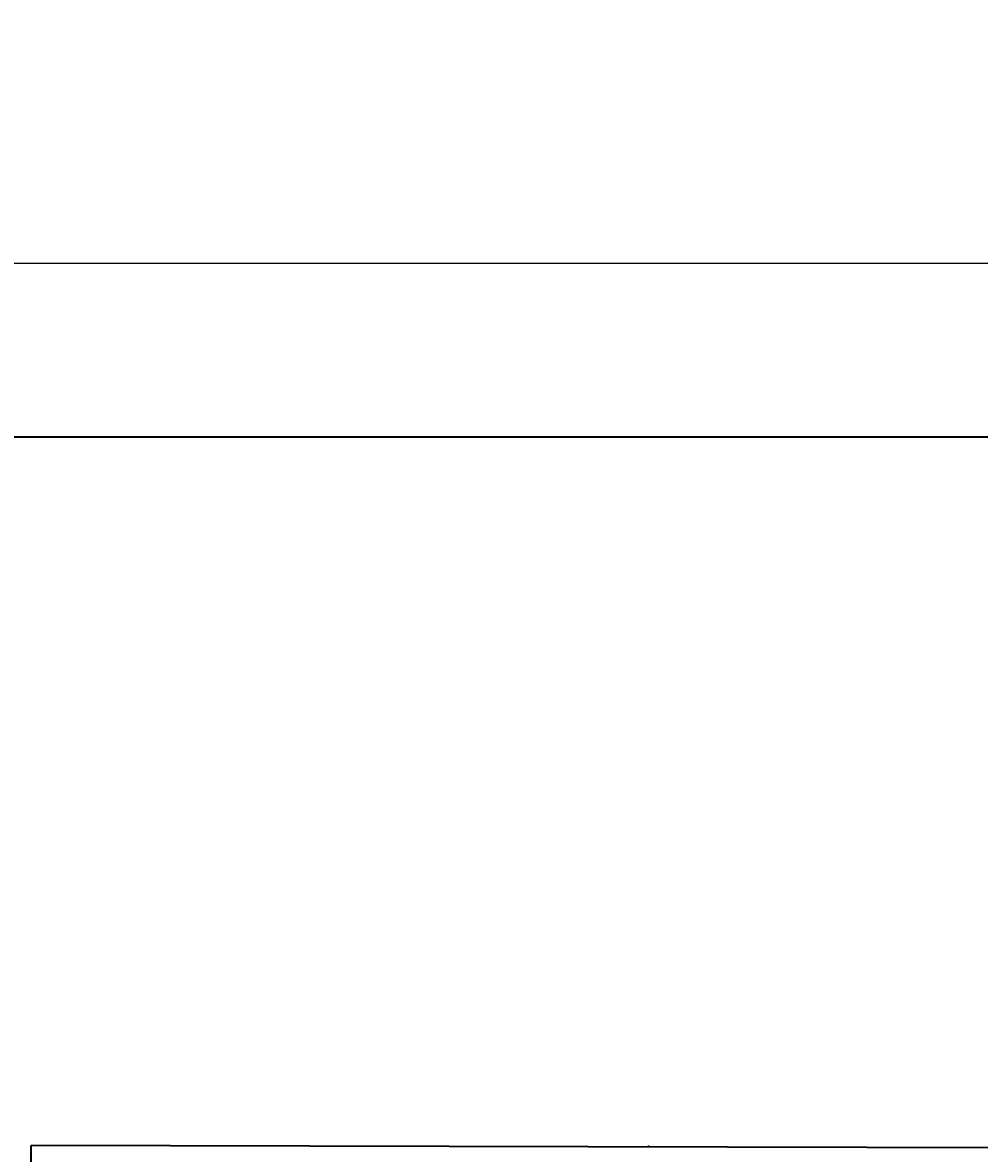
# Model space of a CAD drawing. Units: inches. Extents: x 27 to 200, y -50 to 102.
# Tile 16 of 26: x 89 to 117, y 19 to 52. Entities that reach past the tile are written whole.
import ezdxf

# ---------------------------------------------------------------- set-up
doc = ezdxf.new("R2010")
doc.units = ezdxf.units.IN
doc.header["$MEASUREMENT"] = 0
doc.layers.add('A-ANNO-DIMS', color=2, linetype='Continuous', lineweight=18)
doc.layers.add('A-ELEV', color=7, linetype='Continuous', lineweight=35)
doc.styles.get("Standard").update_dxf_attribs({"font": 'arial.ttf'})
doc.dimstyles.get("Standard").update_dxf_attribs({"dimtxt": 0.18, "dimasz": 0.18, "dimexe": 0.18, "dimexo": 0.0625, "dimgap": 0.09, "dimtad": 0, "dimtih": 1, "dimtoh": 1, "dimdec": 4, "dimzin": 0, "dimdsep": 46, "dimtxsty": 'Standard', "dimcen": 0.09, "dimadec": 0, "dimazin": 0, "dimtfac": 1, "dimtdec": 4, "dimtofl": 0, "dimtmove": 0, "dimatfit": 3, "dimfxl": 1, "dimtolj": 1, "dimtzin": 0, "dimarcsym": 0})

# ---------------------------------------------------------------- blocks, each defined once
blk = doc.blocks.new('*D48')
at = {"layer": 'A-ANNO-DIMS', "color": 0, "lineweight": -2, "transparency": 16777216}
for p, q in [((84.479, 44.926), (199.797, 44.926)), ((199.617, 44.746), (199.617, 14.26)), ((199.617, -16.589), (199.617, 13.897)), ((84.479, -16.769), (199.797, -16.769))]:
    blk.add_line(p, q, dxfattribs=at)
at = {"layer": 'A-ANNO-DIMS', "color": 0, "transparency": 16777216}
for points in [[(199.587, 44.746), (199.647, 44.746), (199.617, 44.926)], [(199.587, -16.589), (199.647, -16.589), (199.617, -16.769)]]:
    blk.add_solid(points, dxfattribs=at)
at = {"layer": 'Defpoints', "color": 0, "transparency": 16777216}
for p in [(84.417, 44.926), (199.617, 44.926), (84.417, -16.769)]:
    blk.add_point(p, dxfattribs=at)
at = {"layer": 'A-ANNO-DIMS', "color": 0, "transparency": 16777216, "insert": (199.617, 14.079), "char_height": 0.18, "attachment_point": 5}
blk.add_mtext('\\A1;61.7', dxfattribs=at)

msp = doc.modelspace()

# ---------------------------------------------------------------- linework, layer by layer
at = {"layer": 'A-ELEV'}
for p, q in [((89.3118, -16.7693), (89.3118, 19.2307)), ((191.4169, 19.002), (89.3118, 19.2307)), ((98.3118, 19.2105), (98.3118, 19.2307)), ((107.3118, 19.1904), (107.3118, 19.2307))]:
    msp.add_line(p, q, dxfattribs=at)
msp.add_lwpolyline([(84.4169, 65.5865), (120.4169, 65.5865), (120.4169, 39.8559), (84.4169, 39.8559)], close=True, dxfattribs=at)

# ---------------------------------------------------------------- dimensions: what is measured, and where the dimension line sits
at = {"layer": 'A-ANNO-DIMS'}
dim = msp.add_linear_dim(base=(199.6169, 44.9264), p1=(84.4169, -16.7693), p2=(84.4169, 44.9264), angle=90, dimstyle='Standard', override={"dimdec": 1, "dimlfac": 1, "dimrnd": 0, "dimzin": 0, "dimdsep": 46, "dimlunit": 2}, dxfattribs=at)
dim.commit()
dim.dimension.update_dxf_attribs({"geometry": '*D48', "text_midpoint": (199.6169, 14.0786)})

doc.saveas('drawing.dxf')
